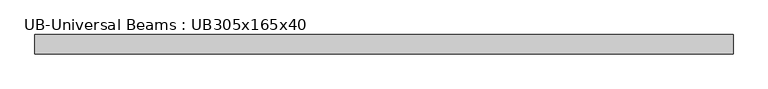
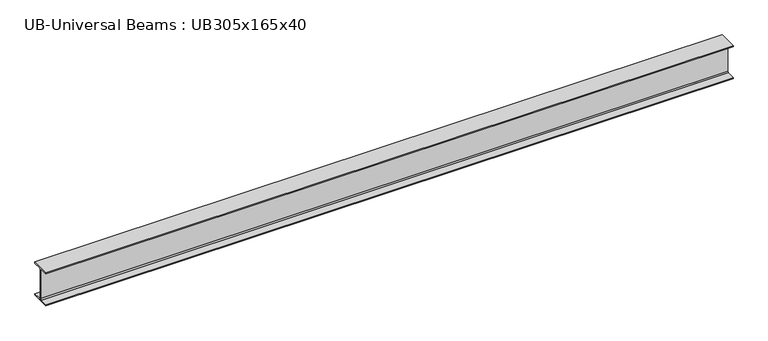
"""IFC4 building model written with IfcOpenShell, lengths in millimetres: beam geometry, UB-Universal Beams : UB305x165x40."""

from ifc_helpers import new_model, si_unit, point, frame, frame_2d, origin, place, context, project, spatial, polyline, circle_curve, trimmed, segment, composite_curve, outline, extrude, source, transform, mapped, element, save


def ub_universal_beams_ub305x165x40_f15b2736(model_context):
    return source(origin(), model_context, "Body", "SweptSolid", [
        extrude(outline(composite_curve([segment(polyline([(82.5, -141.5), (82.5, -151.7), (-82.5, -151.7), (-82.5, -141.5), (-11.9, -141.5)]), True, "CONTINUOUS"), segment(trimmed(circle_curve(frame_2d((-11.9, -132.6)), 8.9), [point((-11.9, -141.5))], [point((-3.0, -132.6))], True, "CARTESIAN"), True, "CONTINUOUS"), segment(polyline([(-3.0, -132.6), (-3.0, 132.6)]), True, "CONTINUOUS"), segment(trimmed(circle_curve(frame_2d((-11.9, 132.6)), 8.9), [point((-3.0, 132.6))], [point((-11.9, 141.5))], True, "CARTESIAN"), True, "CONTINUOUS"), segment(polyline([(-11.9, 141.5), (-82.5, 141.5), (-82.5, 151.7), (82.5, 151.7), (82.5, 141.5), (11.9, 141.5)]), True, "CONTINUOUS"), segment(trimmed(circle_curve(frame_2d((11.9, 132.6)), 8.9), [point((11.9, 141.5))], [point((3.0, 132.6))], True, "CARTESIAN"), True, "CONTINUOUS"), segment(polyline([(3.0, 132.6), (3.0, -132.6)]), True, "CONTINUOUS"), segment(trimmed(circle_curve(frame_2d((11.9, -132.6)), 8.9), [point((3.0, -132.6))], [point((11.9, -141.5))], True, "CARTESIAN"), True, "CONTINUOUS"), segment(polyline([(11.9, -141.5), (82.5, -141.5)]), True, "CONTINUOUS")], self_intersect=False)), frame((-2977.95, 0.0, 0.0), z_axis=(1.0, 0.0, 0.0), x_axis=(0.0, 1.0, 0.0)), (0.0, 0.0, 1.0), 5987.7),
    ])


if __name__ == "__main__":
    model = new_model("IFC4")
    model_context = context("Model", 3, world=origin())
    ifc_project = project(units=[si_unit("LENGTHUNIT", "METRE", prefix="MILLI")], contexts=[model_context])
    site = spatial("IfcSite", under=ifc_project)
    building = spatial("IfcBuilding", under=site)
    placement = place(None, origin())
    ub_universal_beams_ub305x165x40_shape = ub_universal_beams_ub305x165x40_f15b2736(model_context)
    element("IfcBeam", 1, ObjectType="UB-Universal Beams : UB305x165x40", at=placement, inside=building, context=model_context, shape_type="MappedRepresentation", body=[
        mapped(ub_universal_beams_ub305x165x40_shape, transform((0.0, 0.0, 0.0), x_axis=(1.0, 0.0, 0.0), y_axis=(0.0, 1.0, 0.0), z_axis=(0.0, 0.0, 1.0))),
    ])
    save(model, "model.ifc")

# Revit data of these elements
# Type "UB-Universal Beams : UB305x165x40"
#   Section Name Key = "UB305X165X40"
#   Width = 16.5 cm
#   Web Thickness = 0.6 cm
#   Web Fillet = 0.89 cm
#   Warping Constant = 164000.0 cm⁶
#   Torsional Moment of Inertia = 14.70 cm⁴
#   Section Area = 51.3 cm²
#   Plastic Modulus weak axis = 142.0 cm³
#   Plastic Modulus strong axis = 623.0 cm³
#   Nominal Weight = 40.2999 kgf/m
#   Moment of Inertia weak axis = 764.00 cm⁴
#   Moment of Inertia strong axis = 8503.00 cm⁴
#   Height = 30.34 cm
#   Flange Thickness = 1.02 cm
#   Elastic Modulus weak axis = 92.6 cm³
#   Elastic Modulus strong axis = 560.0 cm³
#   Centroid Vertical = 15.17 cm
#   Centroid Horizontal = 8.25 cm
#   Bolt Spacing = 9.0 cm
#   Length [instance default] = 1500 mm
#   Structural Material [instance default] = Metal - Steel 43-275
#   Type Comments = ""
#   Assembly Code = ""
# Element 1 (IfcBeam, "UB-Universal Beams : UB305x165x40")
#   Materials on its faces: "Metal - Steel 43-275"
# Materials
#   "Metal - Steel 43-275": class "Metal", colour RGB 247 247 247, transparency 0, Cost = 0
